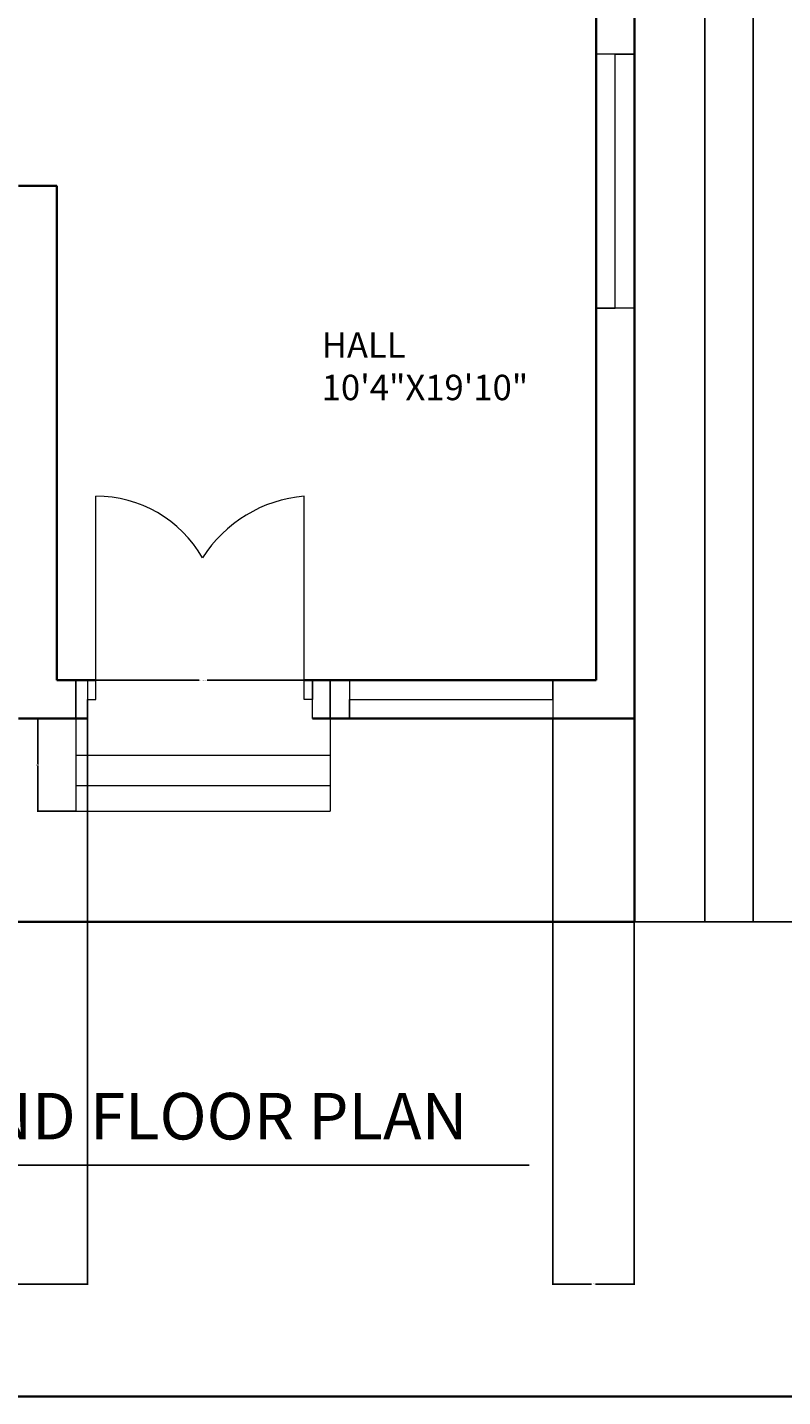
# Model space of a CAD drawing. Units: inches. Extents: x 1911 to 3278, y 2022 to 3108.
# Tile 7 of 13: x 2120 to 2298, y 2022 to 2345. Entities that reach past the tile are written whole.
import ezdxf

# ---------------------------------------------------------------- set-up
doc = ezdxf.new("R2010")
doc.units = ezdxf.units.IN
for name, color, linetype, lineweight in [('A-ANNO-DIMS', 2, 'Continuous', 18), ('A-ANNO-TITL', 7, 'Continuous', 25), ('A-ANNO-TTLB', 7, 'Continuous', 35), ('A-AREA-IDEN', 7, 'Continuous', 18), ('A-DOOR', 4, 'Continuous', 18), ('A-FLOR-STRS', 7, 'Continuous', 18), ('A-GLAZ', 4, 'Continuous', 18), ('A-WALL', 7, 'Continuous', 35)]:
    doc.layers.add(name, color=color, linetype=linetype, lineweight=lineweight)
doc.styles.get("Standard").update_dxf_attribs({"font": 'arial.ttf'})
doc.dimstyles.get("Standard").update_dxf_attribs({"dimtxt": 0.18, "dimasz": 0.18, "dimexe": 0.18, "dimexo": 0.0625, "dimgap": 0.09, "dimtad": 0, "dimtih": 1, "dimtoh": 1, "dimdec": 4, "dimzin": 0, "dimdsep": 46, "dimtxsty": 'Standard', "dimcen": 0.09, "dimadec": 0, "dimazin": 0, "dimtfac": 1, "dimtdec": 4, "dimtofl": 0, "dimtmove": 0, "dimatfit": 3, "dimfxl": 1, "dimtolj": 1, "dimtzin": 0, "dimarcsym": 0})

# ---------------------------------------------------------------- blocks, each defined once
blk = doc.blocks.new('WIN-60')
for p, q in [((0, 60), (9, 60)), ((9, 60), (4.5, 60)), ((4.5, 60), (4.5, 0)), ((4.5, 0), (0, 0)), ((0, 0), (9, 0))]:
    blk.add_line(p, q)
blk = doc.blocks.new('WIN-48')
for p, q in [((0, 9), (0, 0)), ((48, 4.5), (48, 9)), ((48, 9), (48, 0)), ((0, 0), (0, 4.5)), ((0, 4.5), (36, 4.5)), ((36, 4.5), (48, 4.5))]:
    blk.add_line(p, q)
blk = doc.blocks.new('DOOR-ENTRY-PAIR')
for p, q in [((2, 40.5), (2, 52.5)), ((51.21, 4.5), (51.21, 52.5)), ((2, 4.5), (2, 40.5)), ((0, 9), (0, 0)), ((53.21, 0), (53.21, 9)), ((53.21, 9), (53.21, 4.5)), ((0, 0), (0, 4.5)), ((0, 4.5), (2, 4.5)), ((53.21, 4.5), (51.21, 4.5))]:
    blk.add_line(p, q)
for centre, radius, start, end in [((2, 23.47), 29.03, 29.8191, 90), ((54.01, 20.81), 31.81, 95.0534, 147.4925)]:
    blk.add_arc(centre, radius, start, end)
blk = doc.blocks.new('STEPS-ENTRY')
for p, q in [((0, 21.91), (0, 0)), ((60.1, 21.91), (60.1, 0)), ((0, 13.22), (60.1, 13.22)), ((60.1, 13.22), (60.1, 6)), ((60.1, 6), (0, 6)), ((0, 6), (0, 0)), ((0, 0), (60.1, 0))]:
    blk.add_line(p, q)
blk = doc.blocks.new('*D56')
at = {"layer": 'A-ANNO-DIMS', "color": 0, "lineweight": -2, "transparency": 16777216}
for p, q in [((2131.39, 2181.94), (2131.39, 2191.07)), ((2131.57, 2190.89), (2160.46, 2190.89)), ((2191.31, 2190.89), (2162.41, 2190.89)), ((2191.49, 2181.94), (2191.49, 2191.07))]:
    blk.add_line(p, q, dxfattribs=at)
at = {"layer": 'A-ANNO-DIMS', "color": 0, "transparency": 16777216}
for points in [[(2131.57, 2190.92), (2131.57, 2190.86), (2131.39, 2190.89)], [(2191.31, 2190.92), (2191.31, 2190.86), (2191.49, 2190.89)]]:
    blk.add_solid(points, dxfattribs=at)
at = {"layer": 'Defpoints', "color": 0, "transparency": 16777216}
for p in [(2191.49, 2190.89), (2131.39, 2181.87), (2191.49, 2181.87)]:
    blk.add_point(p, dxfattribs=at)
at = {"layer": 'A-ANNO-DIMS', "color": 0, "transparency": 16777216, "insert": (2161.44, 2190.89), "char_height": 0.18, "attachment_point": 5}
blk.add_mtext('\\A1;STEPS 60 TYP.', dxfattribs=at)
blk = doc.blocks.new('*D57')
at = {"layer": 'A-ANNO-DIMS', "color": 0, "lineweight": -2, "transparency": 16777216}
for p, q in [((2131.33, 2181.87), (2122.19, 2181.87)), ((2122.37, 2181.69), (2122.37, 2171.1)), ((2122.37, 2160.15), (2122.37, 2170.74)), ((2131.33, 2159.97), (2122.19, 2159.97))]:
    blk.add_line(p, q, dxfattribs=at)
at = {"layer": 'A-ANNO-DIMS', "color": 0, "transparency": 16777216}
for points in [[(2122.34, 2181.69), (2122.4, 2181.69), (2122.37, 2181.87)], [(2122.34, 2160.15), (2122.4, 2160.15), (2122.37, 2159.97)]]:
    blk.add_solid(points, dxfattribs=at)
at = {"layer": 'Defpoints', "color": 0, "transparency": 16777216}
for p in [(2122.37, 2181.87), (2131.39, 2181.87), (2131.39, 2159.97)]:
    blk.add_point(p, dxfattribs=at)
at = {"layer": 'A-ANNO-DIMS', "color": 0, "transparency": 16777216, "insert": (2122.37, 2170.92), "char_height": 0.18, "attachment_point": 5}
blk.add_mtext('\\A1;22 TYP.', dxfattribs=at)
blk = doc.blocks.new('*D67')
at = {"layer": 'A-ANNO-DIMS', "color": 0, "lineweight": -2, "transparency": 16777216}
for p, q in [((2263.4, 2620.87), (2291.61, 2620.87)), ((2291.43, 2620.69), (2291.43, 2377.56)), ((2291.43, 2134.05), (2291.43, 2377.19)), ((2263.4, 2133.87), (2291.61, 2133.87))]:
    blk.add_line(p, q, dxfattribs=at)
at = {"layer": 'A-ANNO-DIMS', "color": 0, "transparency": 16777216}
for points in [[(2291.4, 2620.69), (2291.46, 2620.69), (2291.43, 2620.87)], [(2291.4, 2134.05), (2291.46, 2134.05), (2291.43, 2133.87)]]:
    blk.add_solid(points, dxfattribs=at)
at = {"layer": 'Defpoints', "color": 0, "transparency": 16777216}
for p in [(2263.33, 2620.87), (2291.43, 2620.87), (2263.33, 2133.87)]:
    blk.add_point(p, dxfattribs=at)
at = {"layer": 'A-ANNO-DIMS', "color": 0, "transparency": 16777216, "insert": (2291.43, 2377.37), "char_height": 0.18, "attachment_point": 5}
blk.add_mtext('\\A1;487', dxfattribs=at)
blk = doc.blocks.new('*D70')
at = {"layer": 'A-ANNO-DIMS', "color": 0, "lineweight": -2, "transparency": 16777216}
for p, q in [((2134.1, 2181.81), (2134.1, 2048.12)), ((2016.83, 2133.81), (2016.83, 2048.12)), ((2017.01, 2048.3), (2075.01, 2048.3)), ((2133.92, 2048.3), (2075.92, 2048.3))]:
    blk.add_line(p, q, dxfattribs=at)
at = {"layer": 'A-ANNO-DIMS', "color": 0, "transparency": 16777216}
for points in [[(2017.01, 2048.33), (2017.01, 2048.27), (2016.83, 2048.3)], [(2133.92, 2048.33), (2133.92, 2048.27), (2134.1, 2048.3)]]:
    blk.add_solid(points, dxfattribs=at)
at = {"layer": 'Defpoints', "color": 0, "transparency": 16777216}
for p in [(2134.1, 2181.87), (2016.83, 2133.87), (2134.1, 2048.3)]:
    blk.add_point(p, dxfattribs=at)
at = {"layer": 'A-ANNO-DIMS', "color": 0, "transparency": 16777216, "insert": (2075.47, 2048.3), "char_height": 0.18, "attachment_point": 5}
blk.add_mtext('\\A1;117.27', dxfattribs=at)
blk = doc.blocks.new('*D71')
at = {"layer": 'A-ANNO-DIMS', "color": 0, "lineweight": -2, "transparency": 16777216}
for p, q in [((2244.04, 2181.81), (2244.04, 2048.12)), ((2263.33, 2133.81), (2263.33, 2048.12)), ((2244.22, 2048.3), (2253.23, 2048.3)), ((2263.15, 2048.3), (2254.14, 2048.3))]:
    blk.add_line(p, q, dxfattribs=at)
at = {"layer": 'A-ANNO-DIMS', "color": 0, "transparency": 16777216}
for points in [[(2244.22, 2048.33), (2244.22, 2048.27), (2244.04, 2048.3)], [(2263.15, 2048.33), (2263.15, 2048.27), (2263.33, 2048.3)]]:
    blk.add_solid(points, dxfattribs=at)
at = {"layer": 'Defpoints', "color": 0, "transparency": 16777216}
for p in [(2244.04, 2181.87), (2263.33, 2133.87), (2263.33, 2048.3)]:
    blk.add_point(p, dxfattribs=at)
at = {"layer": 'A-ANNO-DIMS', "color": 0, "transparency": 16777216, "insert": (2253.69, 2048.3), "char_height": 0.18, "attachment_point": 5}
blk.add_mtext('\\A1;19.294', dxfattribs=at)
blk = doc.blocks.new('*D76')
at = {"layer": 'A-ANNO-DIMS', "color": 0, "lineweight": -2, "transparency": 16777216}
for p, q in [((2308.06, 2620.87), (2279.84, 2620.87)), ((2280.02, 2620.69), (2280.02, 2377.56)), ((2280.02, 2134.05), (2280.02, 2377.19)), ((2308.06, 2133.87), (2279.84, 2133.87))]:
    blk.add_line(p, q, dxfattribs=at)
at = {"layer": 'A-ANNO-DIMS', "color": 0, "transparency": 16777216}
for points in [[(2279.99, 2620.69), (2280.05, 2620.69), (2280.02, 2620.87)], [(2279.99, 2134.05), (2280.05, 2134.05), (2280.02, 2133.87)]]:
    blk.add_solid(points, dxfattribs=at)
at = {"layer": 'Defpoints', "color": 0, "transparency": 16777216}
for p in [(2280.02, 2620.87), (2308.12, 2620.87), (2308.12, 2133.87)]:
    blk.add_point(p, dxfattribs=at)
at = {"layer": 'A-ANNO-DIMS', "color": 0, "transparency": 16777216, "insert": (2280.02, 2377.37), "char_height": 0.18, "attachment_point": 5}
blk.add_mtext('\\A1;487', dxfattribs=at)

msp = doc.modelspace()

# ---------------------------------------------------------------- linework, layer by layer
at = {"layer": 'A-ANNO-TITL'}
msp.add_line((2065.2731, 2076.4043), (2238.4413, 2076.4043), dxfattribs=at)
at = {"layer": 'A-ANNO-TTLB'}
msp.add_lwpolyline([(1911.3875, 3108.0628), (3278.3142, 3108.0628), (3278.3142, 2021.7237), (1911.3875, 2021.7237)], close=True, dxfattribs=at)
at = {"layer": 'A-WALL'}
for p, q in [((2263.3344, 2620.8733), (2263.3344, 2133.8733)), ((2254.3344, 2611.8733), (2254.3344, 2226.8733)), ((2126.8344, 2307.6624), (2117.8344, 2307.6624)), ((2126.8344, 2272.8733), (2126.8344, 2307.6624)), ((2126.8344, 2272.8733), (2126.8344, 2226.8733)), ((2126.8344, 2190.8733), (2126.8344, 2226.8733)), ((2254.3344, 2226.8733), (2254.3344, 2190.8733)), ((2136.1034, 2190.8733), (2126.8344, 2190.8733)), ((2185.3146, 2190.8733), (2254.3344, 2190.8733)), ((2117.8344, 2181.8733), (2134.1034, 2181.8733)), ((2187.3146, 2181.8733), (2263.3344, 2181.8733)), ((2016.8344, 2133.8733), (2126.8344, 2133.8733)), ((2126.8344, 2133.8733), (2263.3344, 2133.8733))]:
    msp.add_line(p, q, dxfattribs=at)

# ---------------------------------------------------------------- block references
at = {"layer": 'A-DOOR'}
msp.add_blockref('DOOR-ENTRY-PAIR', (2134.103, 2181.873), dxfattribs=at)
at = {"layer": 'A-FLOR-STRS'}
msp.add_blockref('STEPS-ENTRY', (2131.388, 2159.968), dxfattribs=at)
at = {"layer": 'A-GLAZ', "rotation": 180}
msp.add_blockref('WIN-60', (2263.3348, 2338.712), dxfattribs=at)
at = {"layer": 'A-GLAZ'}
msp.add_blockref('WIN-48', (2196.041, 2181.873), dxfattribs=at)

# ---------------------------------------------------------------- texts
at = {"layer": 'A-ANNO-TITL', "insert": (2068.3363, 2093.4469), "char_height": 11, "attachment_point": 1}
msp.add_mtext_dynamic_manual_height_columns('GROUND FLOOR PLAN', width=300.572415, gutter_width=12.5, heights=[0], dxfattribs=at)
at = {"layer": 'A-AREA-IDEN', "insert": (2189.4538, 2273.0257), "char_height": 6, "attachment_point": 1}
msp.add_mtext_dynamic_manual_height_columns('HALL\\P10\'4"X19\'10"', width=120.520861, gutter_width=12.5, heights=[0], dxfattribs=at)

# ---------------------------------------------------------------- dimensions: what is measured, and where the dimension line sits
at = {"layer": 'A-ANNO-DIMS'}
for base, p1, p2, picture, middle in [((2291.4344, 2620.8733), (2263.3344, 2133.8733), (2263.3344, 2620.8733), '*D67', (2291.4344, 2377.3733)), ((2280.0192, 2620.8733), (2308.1192, 2133.8733), (2308.1192, 2620.8733), '*D76', (2280.0192, 2377.3733))]:
    dim = msp.add_linear_dim(base=base, p1=p1, p2=p2, angle=90, dimstyle='Standard', override={"dimdec": 0, "dimlfac": 1, "dimrnd": 0, "dimzin": 0, "dimdsep": 46, "dimlunit": 2}, dxfattribs=at)
    dim.commit()
    dim.dimension.update_dxf_attribs({"geometry": picture, "text_midpoint": middle})
dim = msp.add_linear_dim(base=(2191.4893, 2190.8886), p1=(2131.3876, 2181.8733), p2=(2191.4893, 2181.8733), text='STEPS <> TYP.', dimstyle='Standard', override={"dimdec": 0, "dimlfac": 1, "dimrnd": 0, "dimzin": 0, "dimdsep": 46, "dimlunit": 2}, dxfattribs=at)
dim.commit()
dim.dimension.update_dxf_attribs({"geometry": '*D56', "text_midpoint": (2161.4384, 2190.8886)})
for base, p1, p2, override, picture, middle in [((2134.1034, 2048.3043), (2016.8344, 2133.8733), (2134.1034, 2181.8733), {"dimdec": 2, "dimlfac": 1, "dimrnd": 0, "dimzin": 0, "dimdsep": 46, "dimlunit": 2}, '*D70', (2075.4689, 2048.3043)), ((2263.3344, 2048.3043), (2244.0406, 2181.8733), (2263.3344, 2133.8733), {"dimdec": 3, "dimlfac": 1, "dimrnd": 0, "dimzin": 0, "dimdsep": 46, "dimlunit": 2}, '*D71', (2253.6875, 2048.3043))]:
    dim = msp.add_linear_dim(base=base, p1=p1, p2=p2, dimstyle='Standard', override=override, dxfattribs=at)
    dim.commit()
    dim.dimension.update_dxf_attribs({"geometry": picture, "text_midpoint": middle})
dim = msp.add_linear_dim(base=(2122.3723, 2181.8733), p1=(2131.3876, 2159.968), p2=(2131.3876, 2181.8733), angle=90, text='<> TYP.', dimstyle='Standard', override={"dimdec": 0, "dimlfac": 1, "dimrnd": 0, "dimzin": 0, "dimdsep": 46, "dimlunit": 2}, dxfattribs=at)
dim.commit()
dim.dimension.update_dxf_attribs({"geometry": '*D57', "text_midpoint": (2122.3723, 2170.9206)})

doc.saveas('drawing.dxf')
